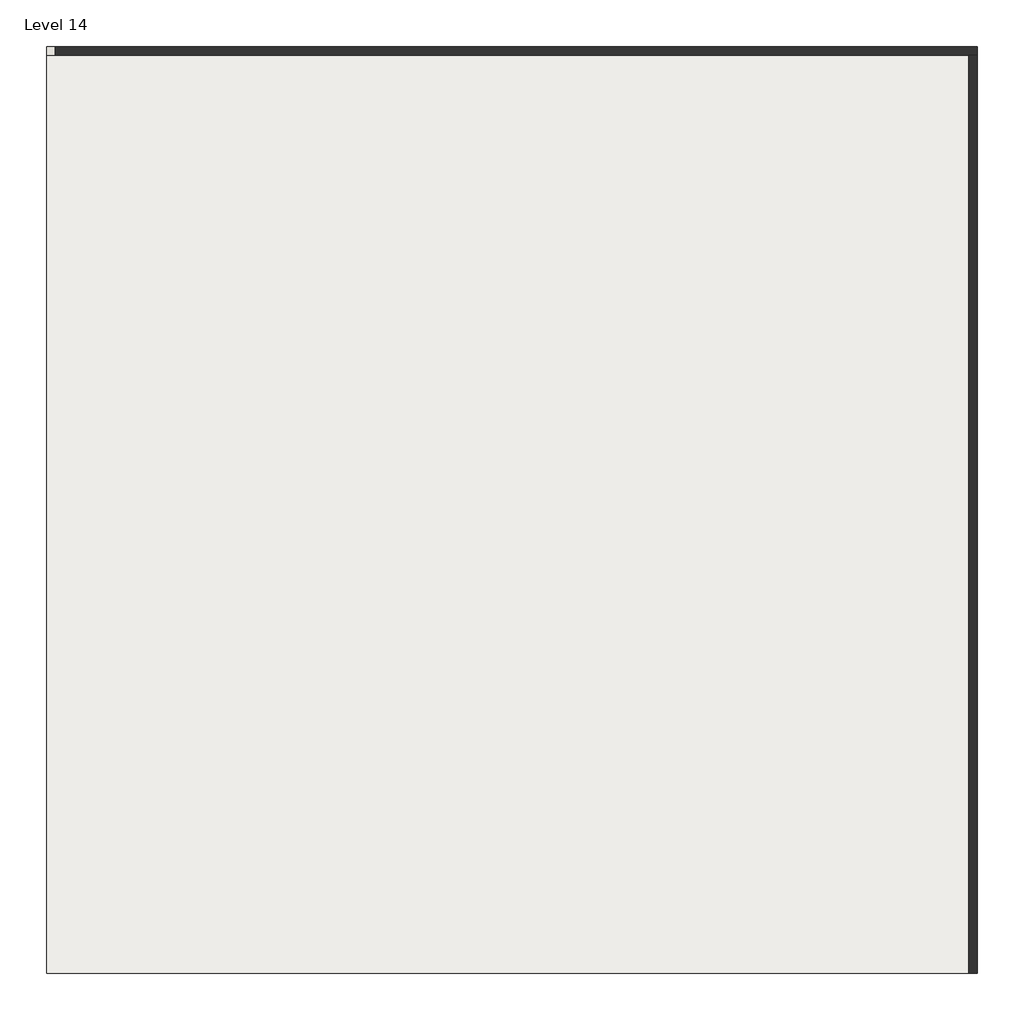
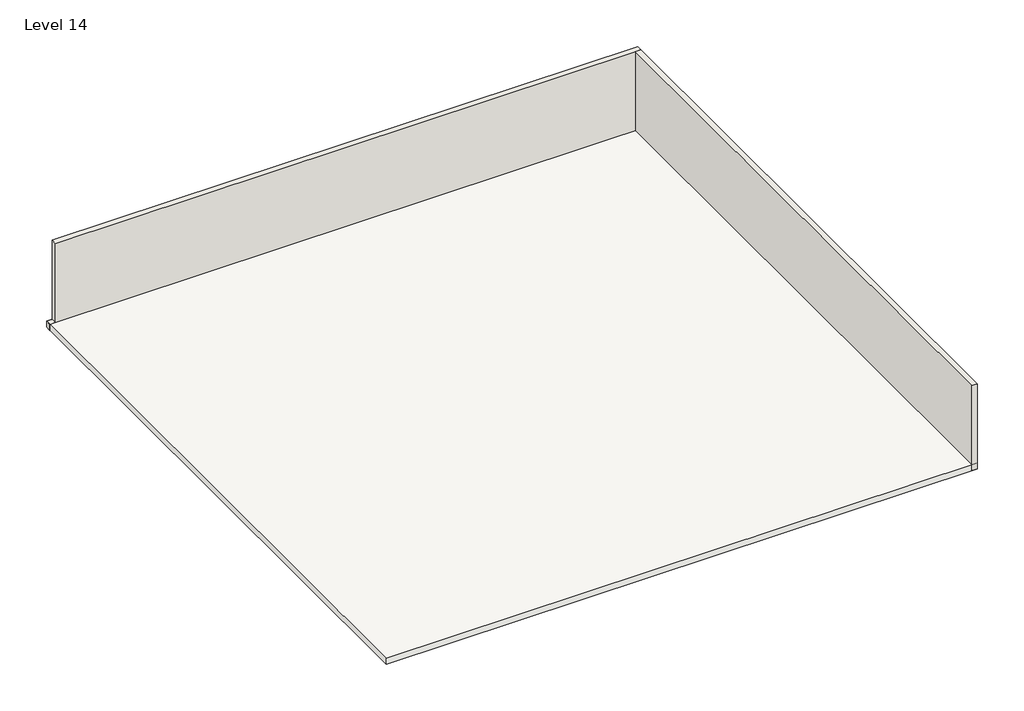
# One storey: 2 walls, 1 roof.
"""IFC4 building model written with IfcOpenShell, lengths in millimetres."""

from ifc_helpers import new_model, si_unit, frame, origin, place, context, project, spatial, polyline, outline, extrude, faceted_brep, element, save

model = new_model("IFC4")

# Units and contexts
model_context = context("Model", 3, world=origin())
ifc_project = project(units=[si_unit("LENGTHUNIT", "METRE", prefix="MILLI")], contexts=[model_context])

# Site, building, storey
site = spatial("IfcSite", under=ifc_project)
building = spatial("IfcBuilding", under=site)
storey = spatial("IfcBuildingStorey", under=building, Name="Level 14", Elevation=22707.6)

# Roof
placement = place(None, origin())
element("IfcRoof", 1, ObjectType="Generic - 9\"", at=placement, inside=storey, context=model_context, shape_type="SweptSolid", body=[
    extrude(outline(polyline([(-8934.7629849, 17755.0995758), (12604.4370151, 17755.0995758), (12604.4370151, -3682.5004242), (-8934.7629849, -3682.5004242), (-8934.7629849, 17755.0995758)])), frame((0.0, 0.0, 22707.6), z_axis=(0.0, 0.0, 1.0), x_axis=(1.0, 0.0, 0.0)), (0.0, 0.0, 1.0), 228.6),
])

# Walls
element("IfcWall", 2, ObjectType="outer wall", at=placement, inside=storey, context=model_context, shape_type="Brep", body=[
    faceted_brep([(-8934.7629849, 17551.8995758, 22707.6), (-8731.5629849, 17551.8995758, 22707.6), (12401.2370151, 17551.8995758, 22707.6), (12604.4370151, 17551.8995758, 22707.6), (12604.4370151, 17551.8995758, 25984.2), (12401.2370151, 17551.8995758, 25984.2), (-8731.5629849, 17551.8995758, 25984.2), (-8731.5629849, 17551.8995758, 22936.2), (-8934.7629849, 17551.8995758, 22936.2), (-8934.7629849, 17755.0995758, 22707.6), (-8934.7629849, 17755.0995758, 22936.2), (-8731.5629849, 17755.0995758, 22936.2), (-8731.5629849, 17755.0995758, 25984.2), (12604.4370151, 17755.0995758, 25984.2), (12604.4370151, 17755.0995758, 22707.6), (-8731.5629849, 17755.0995758, 22707.6)], [[[0, 1, 2, 3, 4, 5, 6, 7, 8]], [[9, 10, 11, 12, 13, 14, 15]], [[3, 2, 1, 0, 9, 15, 14]], [[6, 5, 4, 13, 12]], [[7, 11, 10, 8]], [[0, 8, 10, 9]], [[7, 6, 12, 11]], [[4, 3, 14, 13]]]),
])
element("IfcWall", 3, ObjectType="outer wall", at=placement, inside=storey, context=model_context, shape_type="SweptSolid", body=[
    extrude(outline(polyline([(12604.4370151, 17551.8995758), (12604.4370151, -3682.5004242), (12401.2370151, -3682.5004242), (12401.2370151, 17551.8995758), (12604.4370151, 17551.8995758)])), frame((0.0, 0.0, 22707.6), z_axis=(0.0, 0.0, 1.0), x_axis=(1.0, 0.0, 0.0)), (0.0, 0.0, 1.0), 3276.6),
])

save(model, "model.ifc")

# Revit data of these elements
# Type "Generic - 9\""
#   Assembly Code = "B1020"
#   Layers, outside or top first: 0' - 9" no material (function 1)
# Type "outer wall"
#   Assembly Code = "B2010"
#   Layers, outside or top first: 0' - 8" "Copper" (function 1)
# Element 1 (IfcRoof, "Generic - 9\"")
#   built-in parameter 1001705 = 75.25 (stored number, unit not read)
#   built-in parameter 1001710 = 33615
#   Phase Created = New Construction
#   Materials on its faces: "Default Roof"
# Elements 2, 3 (IfcWall, "outer wall")
#   Top Offset = 0' - 0"
#   Base Offset = 0' - 0"
#   Unconnected Height = 10' - 9"
#   wall height = 10' - 9"
#   Phase Created = New Construction
#   Base Constraint = Level 14
#   Materials on its faces: "Copper"
# Materials
#   "Copper": class "Metal", colour RGB 0 0 0, transparency 0, Description = "Copper, matte finish", Cost = 0
#   "Default Roof": colour RGB 88 101 114, transparency 0
